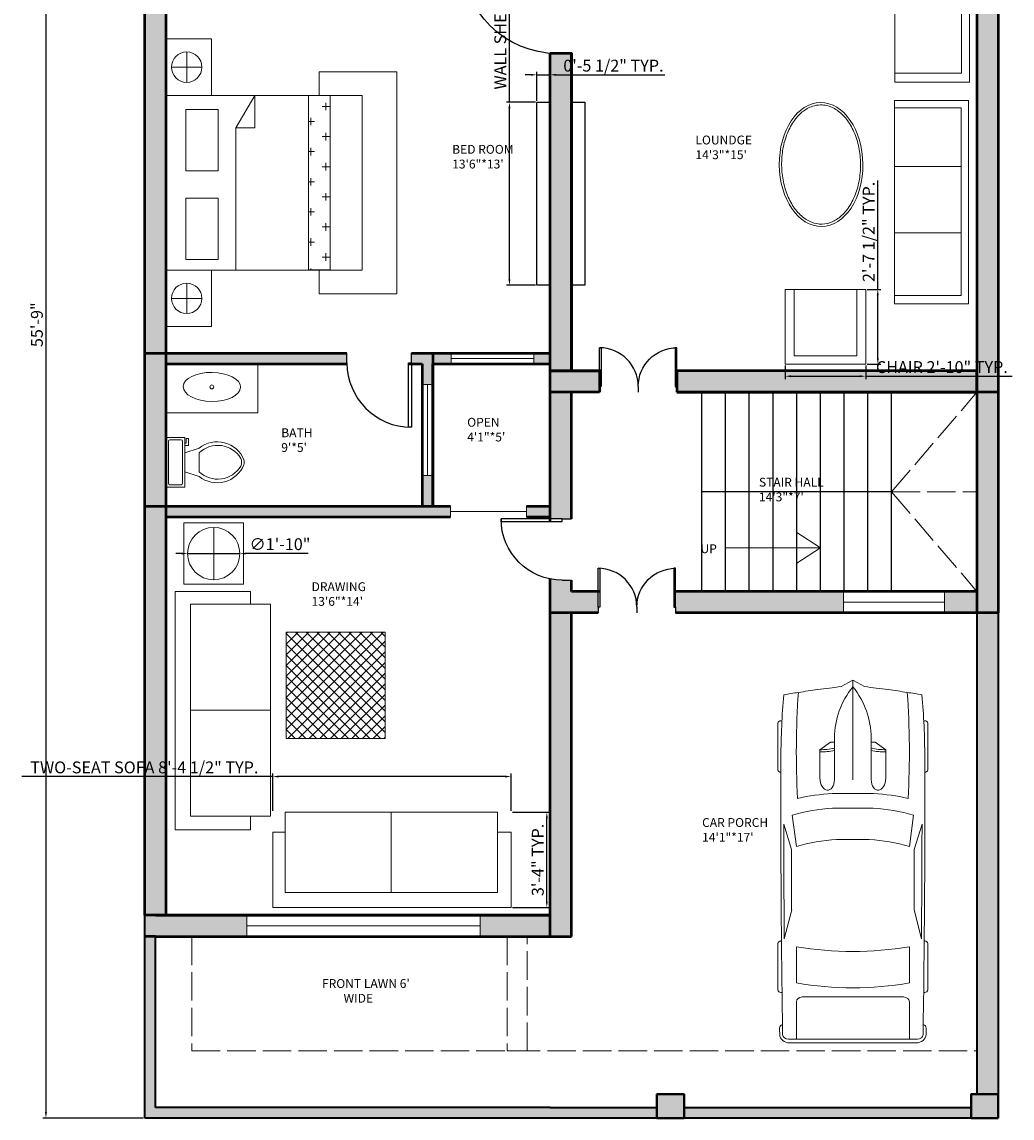
# Model space of a CAD drawing. Units: inches. Extents: x 1864 to 2313, y 963 to 1675.
# Tile 1 of 2: x 1864 to 2282, y 963 to 1425. Entities that reach past the tile are written whole.
import ezdxf

# ---------------------------------------------------------------- set-up
doc = ezdxf.new("R2010")
doc.units = ezdxf.units.IN
doc.linetypes.add('ACAD_ISO02W100', pattern=[15, 12, -3])
for name, color, linetype, lineweight in [('A-ANNO-DIMS', 210, 'Continuous', 18), ('A-ANNO-SYMB', 90, 'Continuous', 18), ('A-AREA-IDEN', 210, 'Continuous', 18), ('A-COLS', 7, 'Continuous', 40), ('A-FLOR-CASE', 230, 'Continuous', 25), ('A-FLOR-FIXT', 40, 'Continuous', 18), ('A-FLOR-OVHD', 142, 'ACAD_ISO02W100', 18), ('A-FLOR-STRS', 90, 'Continuous', 25), ('A-FLOR-STRS-HIDN', 90, 'ACAD_ISO02W100', 18), ('A-FURN-PATT', 40, 'Continuous', 13), ('A-SITE-VEHC', 230, 'Continuous', 13), ('A-SITE-WALL', 7, 'Continuous', 35), ('A-WALL-PATT', 142, 'Continuous', 13), ('door', 50, 'Continuous', 25), ('fur', 40, 'Continuous', 18), ('text', 210, 'Continuous', 18), ('wall', 7, 'Continuous', 50), ('wind', 201, 'Continuous', 20)]:
    doc.layers.add(name, color=color, linetype=linetype, lineweight=lineweight)
doc.styles.get("Standard").update_dxf_attribs({"font": 'arial.ttf'})
doc.dimstyles.new('ISO-25', dxfattribs={"dimtxt": 5, "dimasz": 2.5, "dimexe": 1.25, "dimexo": 0.625, "dimtad": 1, "dimdec": 0, "dimlunit": 4, "dimtxsty": 'Standard', "dimcen": 2.5, "dimadec": 0, "dimazin": 0, "dimtfac": 1, "dimtdec": 0, "dimtmove": 0, "dimatfit": 3, "dimfxl": 1, "dimarcsym": 0})

# ---------------------------------------------------------------- blocks, each defined once
blk = doc.blocks.new('*U6')
for p, q in [((21.1, 37.41), (21.1, 36.83)), ((46.55, 38.89), (22.35, 38.89)), ((47.8, 37.39), (47.8, 37.41)), ((87.99, 31.87), (74.76, 35.92)), ((134.31, 35.6), (119.29, 31.78)), ((135.45, 37.07), (135.45, 37.41)), ((136.7, 38.89), (160.9, 38.89)), ((162.15, 37.41), (162.15, 36.77)), ((70.03, 31.54), (86.41, 29.35)), ((138.42, 29.35), (157.25, 29.35)), ((186.47, 29.35), (167.01, 29.35)), ((186.47, -33.5), (186.47, 33.5)), ((188.4, -32.76), (188.4, 32.76)), ((164.52, 26.39), (164.52, -26.39)), ((32.27, 11.63), (36.13, 17.17)), ((36.13, 17.17), (50.94, 17.17)), ((3.27, 6.13), (0.1, 0.41)), ((29.77, 9.51), (51.68, 9.51)), ((32.12, 9.51), (32.12, 11.15)), ((58.92, -10.77), (58.92, 10.77)), ((66.55, -10.53), (66.55, 10.53)), ((82.74, 8.5), (82.74, -8.5)), ((186.47, -10.53), (186.47, 10.53)), ((0, 0), (51.68, 0)), ((0.1, -0.41), (3.27, -6.13)), ((29.77, -9.51), (51.68, -9.51)), ((32.12, -9.51), (32.12, -11.15)), ((32.27, -11.63), (36.13, -17.17)), ((36.13, -17.17), (50.94, -17.17)), ((86.41, -29.35), (70.03, -31.54)), ((87.99, -31.87), (74.76, -35.92)), ((134.31, -35.6), (119.29, -31.78)), ((157.25, -29.35), (138.42, -29.35)), ((167.01, -29.35), (186.47, -29.35)), ((21.1, -37.41), (21.1, -36.83)), ((46.55, -38.89), (22.35, -38.89)), ((47.8, -37.39), (47.8, -37.41)), ((135.45, -37.07), (135.45, -37.41)), ((136.7, -38.89), (160.9, -38.89)), ((162.15, -37.41), (162.15, -36.77))]:
    blk.add_line(p, q)
for centre, major_axis, ratio, start_param, end_param in [((266.03, -27.52), (0, 313.31), 0.842304, 1.367076, 1.39176), ((41.19, -490.86), (0, 528.23), 0.842304, 0.00281, 0.075598), ((22.35, 37.41), (0, -1.48), 0.842304, 3.141593, 4.712389), ((64.48, -10555.62), (0, 10593.03), 0.842304, -0.013397, 0.002797), ((46.55, 37.41), (0, 1.48), 0.842304, -1.570796, 0), ((64.48, -10555.62), (0, -10591.55), 0.842304, 3.133765, 3.140441), ((136.7, 37.41), (0, -1.48), 0.842304, 3.141593, 4.712389), ((160.9, 37.41), (0, 1.48), 0.842304, -1.570796, 0), ((180.63, 35.84), (0, 2.22), 0.842304, -0.013017, 1.249894), ((64.48, -10556.36), (0, 10595.31), 0.842304, -0.013397, -0.013017), ((183.98, 33.5), (0, -2.96), 0.842304, 1.570796, 3.128196), ((183.98, 32.76), (0, -5.25), 0.842304, 1.570796, 3.128196), ((37.47, -593.96), (0, -623.33), 0.842304, 3.096046, 3.200911), ((134.4, 5.39), (0, -89.78), 0.842304, 4.449482, 4.652344), ((135.29, 5.39), (0, 81.77), 0.842304, 1.245306, 1.50788), ((149.6, 2.8), (0, -79.58), 0.842304, 4.372215, 4.640744), ((95.79, -3666.35), (0, -3698.24), 0.842304, 3.134049, 3.144098), ((17.08, 0), (0, 147.02), 0.842304, 4.511394, 4.913384), ((35.91, 0), (0, 147.02), 0.842304, 4.511394, 4.913384), ((167.01, 26.39), (0, 2.96), 0.842304, 0, 1.570796), ((259.18, -27.52), (0, -305.3), 0.842304, 4.528606, 4.561838), ((-204.49, 52.4), (0, -250.96), 0.842304, 1.385369, 1.434372), ((13.04, 17.01), (0, 27.42), 0.842304, 4.435146, 4.718221), ((14.2, 17.01), (0, 27.42), 0.842304, 4.435146, 4.718221), ((50.79, 13.34), (6.34, -0.36), 0.603834, -1.395552, 1.581315), ((32.75, 11.15), (0, 0.74), 0.842304, 0.879714, 1.570796), ((29.77, -46.66), (0, 56.17), 0.842304, 0, 0.590319), ((0.62, 0), (0, -0.74), 0.842304, 4.131459, 5.293319), ((29.77, 46.66), (0, 56.17), 0.842304, 2.551274, 3.141593), ((-204.49, -52.4), (0, 250.96), 0.842304, -1.434372, -1.385369), ((32.75, -11.15), (0, -0.74), 0.842304, 4.712389, 5.403472), ((13.04, -17.01), (0, -27.42), 0.842304, 1.564964, 1.848039), ((14.2, -17.01), (0, -27.42), 0.842304, 1.564964, 1.848039), ((134.4, -5.39), (0, -89.78), 0.842304, -1.510751, -1.307889), ((135.29, -5.39), (0, -81.77), 0.842304, -1.50788, -1.245306), ((149.6, -2.8), (0, -79.58), 0.842304, -1.499151, -1.230623), ((259.18, 27.52), (0, 305.3), 0.842304, 1.721348, 1.754579), ((266.03, 27.52), (0, 313.31), 0.842304, 1.749832, 1.774517), ((37.47, 593.96), (0, -623.33), 0.842304, -0.059319, 0.045547), ((167.01, -26.39), (0, -2.96), 0.842304, 4.712389, 6.283185), ((95.79, 3666.35), (0, -3698.24), 0.842304, -0.002505, 0.007544), ((183.98, -33.5), (0, 2.96), 0.842304, 3.15499, 4.712389), ((183.98, -32.76), (0, -5.25), 0.842304, 0.013397, 1.570796), ((41.19, 490.86), (0, -528.23), 0.842304, -0.075598, -0.00281), ((22.35, -37.41), (0, 1.48), 0.842304, 1.570796, 3.141593), ((64.48, 10555.62), (0, 10593.03), 0.842304, 3.138796, 3.15499), ((46.55, -37.41), (0, -1.48), 0.842304, 0, 1.570796), ((64.48, 10555.62), (0, -10591.55), 0.842304, 0.001152, 0.007828), ((136.7, -37.41), (0, -1.48), 0.842304, -1.570796, 0), ((160.9, -37.41), (0, 1.48), 0.842304, 3.141593, 4.712389), ((180.63, -35.84), (0, -2.22), 0.842304, -1.249894, 0.013017), ((64.48, 10556.36), (0, 10595.31), 0.842304, 3.15461, 3.15499)]:
    blk.add_ellipse(centre, major_axis=major_axis, ratio=ratio, start_param=start_param, end_param=end_param)
at = {"extrusion": (0, 0, -1)}
blk.add_ellipse((50.79, -13.34), major_axis=(6.34, 0.36), ratio=0.603834, start_param=-1.395552, end_param=1.581315, dxfattribs=at)
blk = doc.blocks.new('*U2')
for p, q in [((0, 0), (0, -6)), ((40, 0), (40, -6))]:
    blk.add_line(p, q)
blk.add_lwpolyline([(0, 0), (0, 40), (1.75, 40), (1.75, 0)], close=True)
blk.add_arc((0, 0), 40, 0, 90)
blk = doc.blocks.new('*U4')
for p, q in [((9.5, -6), (9.5, -2)), ((-10, -8.5), (-8, -8.5)), ((-10, -9.5), (-10, -8.5)), ((-8, -8.5), (-8, -8)), ((-7, -8), (-7, -9.5)), ((-4, -8), (-6, -14)), ((4, -8), (6, -14)), ((-7, -9.5), (-10, -9.5)), ((4, -14), (-4, -14))]:
    blk.add_line(p, q)
blk.add_lwpolyline([(10.5, -8), (10.5, 0), (-10.5, 0), (-10.5, -8)], close=True)
for points in [[(-9.5, -2), (-9.5, -6)], [(8.5, -1), (-8.5, -1)], [(-8.5, -7), (8.5, -7)]]:
    blk.add_lwpolyline(points)
for centre, radius, start, end in [((-8.62, -1.88), 0.884, 81.8699, 188.1301), ((8.62, -1.88), 0.884, 351.8699, 98.1301), ((-8.62, -6.12), 0.884, 171.8699, 278.1301), ((8.62, -6.12), 0.884, 261.8699, 8.1301), ((3.52, -21.58), 12.17, 141.4691, 247.9714), ((4.2, -21.82), 11.33, 136.3677, 238.9468), ((-3.52, -21.58), 12.17, 292.0284, 38.5307), ((-4.2, -21.82), 11.33, 301.053, 43.6321), ((0, -27.88), 4, 245.7318, 294.2682), ((0, -29), 4, 254.8605, 285.1395)]:
    blk.add_arc(centre, radius, start, end)
blk = doc.blocks.new('*D10')
at = {"layer": 'A-ANNO-DIMS', "color": 0, "lineweight": -2, "transparency": 16777216}
for p, q in [((1915.33, 1632.16), (1873.06, 1632.16)), ((1874.31, 1629.66), (1874.31, 965.66)), ((1915.33, 963.16), (1873.06, 963.16))]:
    blk.add_line(p, q, dxfattribs=at)
at = {"layer": 'A-ANNO-DIMS', "color": 0, "lineweight": 100, "transparency": 16777216}
for points in [[(1873.89, 1629.66), (1874.73, 1629.66), (1874.31, 1632.16)], [(1873.89, 965.66), (1874.73, 965.66), (1874.31, 963.16)]]:
    blk.add_solid(points, dxfattribs=at)
at = {"layer": 'Defpoints', "color": 0, "lineweight": 100, "transparency": 16777216}
for p in [(1915.95, 1632.16), (1874.31, 963.16), (1915.95, 963.16)]:
    blk.add_point(p, dxfattribs=at)
at = {"layer": 'A-ANNO-DIMS', "color": 0, "transparency": 16777216, "insert": (1871.13, 1297.66), "char_height": 5, "attachment_point": 5, "rotation": 90}
blk.add_mtext('55\'-9"', dxfattribs=at)
blk = doc.blocks.new('BED-DOUBLE')
for p, q in [((10, 67.81), (70, 67.81)), ((70, 67.81), (70, 59.9)), ((83.6, 59.9), (70, 67.81)), ((70, 59.9), (83.6, 59.9)), ((5, 32.66), (0, 32.66)), ((0, 32.66), (0, 0)), ((10, 32.66), (5, 32.66)), ((83.6, 32.66), (93.6, 32.66)), ((93.6, 32.66), (93.6, 0)), ((0, 0), (93.6, 0))]:
    blk.add_line(p, q)
for points in [[(10, 97.3), (83.6, 97.3), (83.6, 14.55), (10, 14.55)], [(14.44, 88.9), (40.24, 88.9), (40.24, 75.28), (14.44, 75.28)], [(51.82, 88.9), (77.62, 88.9), (77.62, 75.28), (51.82, 75.28)]]:
    blk.add_lwpolyline(points, close=True)
blk = doc.blocks.new('TABLE-BEDSIDE')
for p, q in [((11.93, 4.03), (11.93, 16.85)), ((5.53, 10.44), (18.34, 10.44))]:
    blk.add_line(p, q)
blk.add_lwpolyline([(0, 19.17), (23.88, 19.17), (23.88, 0), (0, 0)], close=True)
blk.add_circle((11.93, 10.44), 6.41)
blk = doc.blocks.new('SOFA-TWO-SEAT')
for p, q in [((0, 0), (0, 100.52)), ((31.78, 100.52), (0, 100.52)), ((31.78, 95.26), (31.78, 100.52)), ((40.15, 50.52), (6.4, 50.52)), ((31.78, 5.79), (31.78, 0)), ((31.78, 0), (0, 0))]:
    blk.add_line(p, q)
blk.add_lwpolyline([(6.4, 95.26), (40.15, 95.26), (40.15, 5.79), (6.4, 5.79)], close=True)
blk = doc.blocks.new('LOUNGE-CHAIR')
for p, q in [((3.79, 31.54), (0, 31.54)), ((0, 31.54), (0, 0)), ((3.79, 3.47), (3.79, 31.54)), ((30.24, 31.54), (33.95, 31.54)), ((33.95, 31.54), (33.95, 0)), ((0, 0), (33.95, 0))]:
    blk.add_line(p, q)
blk.add_lwpolyline([(3.79, 31.54), (30.24, 31.54), (30.24, 3.47), (3.79, 3.47)])
blk = doc.blocks.new('BASIN-OVAL')
blk.add_circle((12.11, 6.1), 0.811)
blk.add_ellipse((12.11, 6.1), major_axis=(12.1, -0.16), ratio=0.504372)
blk = doc.blocks.new('WALL-SHELF')
blk.add_lwpolyline([(0, 77.17), (5.6, 77.17), (5.6, 0), (0, 0)], close=True)
blk = doc.blocks.new('*D24')
at = {"layer": 'A-ANNO-DIMS', "color": 0, "lineweight": -2, "transparency": 16777216}
for p, q in [((1969.95, 1107.15), (1864.18, 1107.15)), ((1969.95, 1092.7), (1969.95, 1108.4)), ((2067.97, 1107.15), (1972.45, 1107.15)), ((2070.47, 1092.7), (2070.47, 1108.4))]:
    blk.add_line(p, q, dxfattribs=at)
at = {"layer": 'A-ANNO-DIMS', "color": 0, "lineweight": 100, "transparency": 16777216}
for points in [[(1972.45, 1107.57), (1972.45, 1106.74), (1969.95, 1107.15)], [(2067.97, 1107.57), (2067.97, 1106.74), (2070.47, 1107.15)]]:
    blk.add_solid(points, dxfattribs=at)
at = {"layer": 'Defpoints', "color": 0, "lineweight": 100, "transparency": 16777216}
for p in [(1969.95, 1107.15), (1969.95, 1092.07), (2070.47, 1092.07)]:
    blk.add_point(p, dxfattribs=at)
at = {"layer": 'A-ANNO-DIMS', "color": 0, "transparency": 16777216, "insert": (1915.81, 1110.36), "char_height": 5, "attachment_point": 5}
blk.add_mtext('TWO-SEAT SOFA 8\'-4 1/2" TYP.', dxfattribs=at)
blk = doc.blocks.new('*D25')
at = {"layer": 'A-ANNO-DIMS', "color": 0, "lineweight": -2, "transparency": 16777216}
for p, q in [((2071.09, 1092.07), (2086.8, 1092.07)), ((2085.55, 1054.43), (2085.55, 1089.57)), ((2071.09, 1051.93), (2086.8, 1051.93))]:
    blk.add_line(p, q, dxfattribs=at)
at = {"layer": 'A-ANNO-DIMS', "color": 0, "lineweight": 100, "transparency": 16777216}
for points in [[(2085.13, 1089.57), (2085.96, 1089.57), (2085.55, 1092.07)], [(2085.13, 1054.43), (2085.96, 1054.43), (2085.55, 1051.93)]]:
    blk.add_solid(points, dxfattribs=at)
at = {"layer": 'Defpoints', "color": 0, "lineweight": 100, "transparency": 16777216}
for p in [(2070.47, 1092.07), (2085.55, 1092.07), (2070.47, 1051.93)]:
    blk.add_point(p, dxfattribs=at)
at = {"layer": 'A-ANNO-DIMS', "color": 0, "transparency": 16777216, "insert": (2082.37, 1072), "char_height": 5, "attachment_point": 5, "rotation": 90}
blk.add_mtext('3\'-4" TYP.', dxfattribs=at)
blk = doc.blocks.new('*D26')
at = {"layer": 'A-ANNO-DIMS', "color": 0, "lineweight": -2, "transparency": 16777216}
for p, q in [((2186.08, 1280.4), (2186.08, 1274.68)), ((2220.03, 1280.4), (2220.03, 1274.68)), ((2188.58, 1275.93), (2217.53, 1275.93)), ((2220.03, 1275.93), (2281.76, 1275.93))]:
    blk.add_line(p, q, dxfattribs=at)
at = {"layer": 'A-ANNO-DIMS', "color": 0, "lineweight": 100, "transparency": 16777216}
for points in [[(2188.58, 1276.35), (2188.58, 1275.52), (2186.08, 1275.93)], [(2217.53, 1276.35), (2217.53, 1275.52), (2220.03, 1275.93)]]:
    blk.add_solid(points, dxfattribs=at)
at = {"layer": 'Defpoints', "color": 0, "lineweight": 100, "transparency": 16777216}
for p in [(2186.08, 1281.02), (2220.03, 1281.02), (2220.03, 1275.93)]:
    blk.add_point(p, dxfattribs=at)
at = {"layer": 'A-ANNO-DIMS', "color": 0, "transparency": 16777216, "insert": (2252.15, 1279.14), "char_height": 5, "attachment_point": 5}
blk.add_mtext('CHAIR 2\'-10" TYP.', dxfattribs=at)
blk = doc.blocks.new('*D27')
at = {"layer": 'A-ANNO-DIMS', "color": 0, "lineweight": -2, "transparency": 16777216}
for p, q in [((2225.13, 1312.56), (2225.13, 1358.53)), ((2220.66, 1312.56), (2226.38, 1312.56)), ((2225.13, 1283.52), (2225.13, 1310.06)), ((2220.66, 1281.02), (2226.38, 1281.02))]:
    blk.add_line(p, q, dxfattribs=at)
at = {"layer": 'A-ANNO-DIMS', "color": 0, "lineweight": 100, "transparency": 16777216}
for points in [[(2224.71, 1310.06), (2225.54, 1310.06), (2225.13, 1312.56)], [(2224.71, 1283.52), (2225.54, 1283.52), (2225.13, 1281.02)]]:
    blk.add_solid(points, dxfattribs=at)
at = {"layer": 'Defpoints', "color": 0, "lineweight": 100, "transparency": 16777216}
for p in [(2220.03, 1312.56), (2225.13, 1312.56), (2220.03, 1281.02)]:
    blk.add_point(p, dxfattribs=at)
at = {"layer": 'A-ANNO-DIMS', "color": 0, "transparency": 16777216, "insert": (2221.92, 1336.8), "char_height": 5, "attachment_point": 5, "rotation": 90}
blk.add_mtext('2\'-7 1/2" TYP.', dxfattribs=at)
blk = doc.blocks.new('*D30')
at = {"layer": 'A-ANNO-DIMS', "color": 0, "lineweight": -2, "transparency": 16777216}
for p, q in [((2069.78, 1391.45), (2069.78, 1471.3)), ((2080.73, 1391.45), (2068.53, 1391.45)), ((2069.78, 1316.78), (2069.78, 1388.95)), ((2080.73, 1314.28), (2068.53, 1314.28))]:
    blk.add_line(p, q, dxfattribs=at)
at = {"layer": 'A-ANNO-DIMS', "color": 0, "lineweight": 100, "transparency": 16777216}
for points in [[(2069.36, 1388.95), (2070.19, 1388.95), (2069.78, 1391.45)], [(2069.36, 1316.78), (2070.19, 1316.78), (2069.78, 1314.28)]]:
    blk.add_solid(points, dxfattribs=at)
at = {"layer": 'Defpoints', "color": 0, "lineweight": 100, "transparency": 16777216}
for p in [(2069.78, 1391.45), (2081.35, 1391.45), (2081.35, 1314.28)]:
    blk.add_point(p, dxfattribs=at)
at = {"layer": 'A-ANNO-DIMS', "color": 0, "transparency": 16777216, "insert": (2066.57, 1432.63), "char_height": 5, "attachment_point": 5, "rotation": 90}
blk.add_mtext('WALL SHELF 6\'-5" TYP.', dxfattribs=at)
blk = doc.blocks.new('*D31')
at = {"layer": 'A-ANNO-DIMS', "color": 0, "lineweight": -2, "transparency": 16777216}
for p, q in [((2078.85, 1403.03), (2076.35, 1403.03)), ((2081.35, 1392.08), (2081.35, 1404.28)), ((2081.35, 1403.03), (2086.95, 1403.03)), ((2086.95, 1392.08), (2086.95, 1404.28)), ((2089.45, 1403.03), (2135.33, 1403.03))]:
    blk.add_line(p, q, dxfattribs=at)
at = {"layer": 'A-ANNO-DIMS', "color": 0, "lineweight": 100, "transparency": 16777216}
for points in [[(2078.85, 1403.44), (2078.85, 1402.61), (2081.35, 1403.03)], [(2089.45, 1403.44), (2089.45, 1402.61), (2086.95, 1403.03)]]:
    blk.add_solid(points, dxfattribs=at)
at = {"layer": 'Defpoints', "color": 0, "lineweight": 100, "transparency": 16777216}
for p in [(2086.95, 1403.03), (2081.35, 1391.45), (2086.95, 1391.45)]:
    blk.add_point(p, dxfattribs=at)
at = {"layer": 'A-ANNO-DIMS', "color": 0, "transparency": 16777216, "insert": (2113.64, 1406.24), "char_height": 5, "attachment_point": 5}
blk.add_mtext('0\'-5 1/2" TYP.', dxfattribs=at)
blk = doc.blocks.new('*D34')
at = {"layer": 'A-ANNO-DIMS', "color": 0, "lineweight": -2, "transparency": 16777216}
for p, q in [((1931.54, 1201.15), (1929.04, 1201.15)), ((1934.04, 1201.15), (1956.09, 1201.15)), ((1984.95, 1201.15), (1958.59, 1201.15))]:
    blk.add_line(p, q, dxfattribs=at)
at = {"layer": 'A-ANNO-DIMS', "color": 0, "lineweight": 100, "transparency": 16777216}
for points in [[(1931.54, 1201.56), (1931.54, 1200.73), (1934.04, 1201.15)], [(1958.59, 1201.56), (1958.59, 1200.73), (1956.09, 1201.15)]]:
    blk.add_solid(points, dxfattribs=at)
at = {"layer": 'Defpoints', "color": 0, "lineweight": 100, "transparency": 16777216}
for p in [(1934.04, 1201.15), (1956.09, 1201.15)]:
    blk.add_point(p, dxfattribs=at)
at = {"layer": 'A-ANNO-DIMS', "color": 0, "transparency": 16777216, "insert": (1973.02, 1204.47), "char_height": 5, "attachment_point": 5, "rotation": 359.9997}
blk.add_mtext('∅1\'-10"', dxfattribs=at)

msp = doc.modelspace()

# ---------------------------------------------------------------- hatches: boundary and pattern name
at = {"layer": 'A-FURN-PATT'}
h = msp.add_hatch(dxfattribs=at)
h.set_pattern_fill('CROSS', color=256, angle=90)
h.set_pattern_definition([(90, (3548.109, -701.066), (-6.35, 6.35), [3.175, -9.525]), (180, (3549.697, -699.4784), (-6.35, -6.35), [3.175, -9.525])])
h.paths.add_polyline_path([(1994.15, 1394.32), (1985.02, 1394.32), (1985.02, 1320.73), (1994.15, 1320.73)])
h = msp.add_hatch(dxfattribs=at)
h.set_pattern_fill('ANSI37', color=256)
h.paths.add_polyline_path([(2017.33, 1167.99), (1975.66, 1167.99), (1975.66, 1123.22), (2017.33, 1123.22)])
at = {"layer": 'A-WALL-PATT'}
h = msp.add_hatch(color=256, dxfattribs=at)
h.dxf.hatch_style = 1
h.paths.add_polyline_path([(1975.95, 1632.16), (1961.64, 1632.16), (1961.64, 1623.16), (1971.45, 1623.16), (1975.95, 1623.16)])
h.paths.add_polyline_path([(2021.79, 1632.16), (1989.45, 1632.16), (1975.95, 1632.16), (1975.95, 1623.16), (1984.95, 1623.16), (1989.45, 1623.16), (2021.79, 1623.16)])
h.paths.add_polyline_path([(2161.95, 1632.16), (2126.93, 1632.16), (2126.93, 1623.16), (2157.45, 1623.16), (2161.95, 1623.16)])
h.paths.add_polyline_path([(2275.95, 1632.16), (2258.45, 1632.16), (2258.45, 1623.16), (2266.95, 1623.16), (2266.95, 1475.18, -0.040334), (2266.95, 1472.91), (2266.95, 1467.16), (2266.95, 1458.16), (2266.95, 1278.16), (2266.95, 1269.16), (2275.95, 1269.16), (2275.95, 1458.16)])
h.paths.add_polyline_path([(2161.95, 1623.16), (2157.45, 1623.16), (2157.45, 1467.16), (2154.26, 1467.16), (2154.26, 1464.16), (2154.26, 1458.16), (2161.95, 1458.16)])
h.paths.add_polyline_path([(2202.62, 1632.16), (2198.67, 1632.16), (2198.67, 1627.01, -0.028105), (2198.46, 1623.16), (2202.62, 1623.16)])
h.paths.add_polyline_path([(2164.34, 1627.01), (2164.34, 1632.16), (2161.95, 1632.16), (2161.95, 1623.16), (2164.34, 1623.16)])
h.paths.add_polyline_path([(1930.16, 1632.16), (1929.45, 1632.16), (1915.95, 1632.16), (1915.95, 1458.16), (1924.95, 1458.16), (1924.95, 1623.16), (1930.16, 1623.16)])
h.paths.add_polyline_path([(1924.95, 1441.66), (1924.95, 1458.16), (1915.95, 1458.16), (1915.95, 1285.66), (1924.95, 1285.66)])
h.paths.add_polyline_path([(2044.94, 1221.16), (2037.45, 1221.16), (1924.95, 1221.16), (1924.95, 1216.66), (2044.94, 1216.66)])
h.paths.add_polyline_path([(2037.45, 1234.15), (2032.95, 1234.15), (2032.95, 1221.16), (2037.45, 1221.16)])
h.paths.add_polyline_path([(2086.95, 1221.16), (2076.95, 1221.16), (2076.95, 1216.66), (2086.95, 1216.66)])
h.paths.add_polyline_path([(2107.14, 1185.16), (2095.95, 1185.16), (2095.95, 1189.94), (2092.08, 1189.94, -0.049915), (2086.95, 1190.46), (2086.95, 1176.16), (2107.14, 1176.16), (2107.14, 1178.61)])
h.paths.add_polyline_path([(2095.95, 1176.16), (2086.95, 1176.16), (2086.95, 1056.16), (2086.95, 1039.66), (2095.95, 1039.66), (2095.95, 1056.16)])
h.paths.add_polyline_path([(2086.95, 1048.66), (2057.44, 1048.66), (2057.44, 1039.66), (2086.95, 1039.66)])
h.paths.add_polyline_path([(1959.08, 1048.66), (1915.95, 1048.66), (1915.95, 1039.66), (1920.45, 1039.66), (1959.08, 1039.66)])
h.paths.add_polyline_path([(1924.95, 1216.66), (1924.95, 1221.16), (1915.95, 1221.16), (1915.95, 1048.66), (1924.95, 1048.66)])
h.paths.add_polyline_path([(1924.95, 1281.16), (1924.95, 1285.66), (1915.95, 1285.66), (1915.95, 1221.16), (1924.95, 1221.16)])
h.paths.add_polyline_path([(2037.45, 1285.66), (2028.44, 1285.66), (2028.44, 1281.58), (2028.44, 1281.16), (2032.95, 1281.16), (2032.95, 1272.41), (2037.45, 1272.41)])
h.paths.add_polyline_path([(2045.26, 1285.66), (2037.45, 1285.66), (2037.45, 1281.16), (2045.26, 1281.16)])
h.paths.add_polyline_path([(2086.95, 1285.66), (2080.03, 1285.66), (2080.03, 1281.16), (2086.95, 1281.16)])
h.paths.add_polyline_path([(2095.95, 1269.16), (2086.95, 1269.16), (2086.95, 1215.79), (2092.08, 1215.79), (2095.95, 1215.79)])
h = msp.add_hatch(color=256, dxfattribs=at)
h.dxf.hatch_style = 1
h.paths.add_polyline_path([(2266.95, 1278.16), (2140.44, 1278.16), (2140.44, 1271.61), (2140.44, 1269.16), (2266.95, 1269.16)])
h.paths.add_polyline_path([(2107.74, 1278.16), (2086.95, 1278.16), (2086.95, 1269.16), (2107.74, 1269.16), (2107.74, 1271.61)])
h.paths.add_polyline_path([(2095.95, 1412.1), (2086.95, 1412.1), (2086.95, 1278.16), (2095.95, 1278.16)])
h = msp.add_hatch(color=256, dxfattribs=at)
h.dxf.hatch_style = 1
h.paths.add_polyline_path([(2131.95, 967.66), (2086.95, 967.66), (1920.45, 967.66), (1920.45, 1039.66), (1915.95, 1039.66), (1915.95, 963.16), (2086.95, 963.16), (2131.95, 963.16)])
h.paths.add_polyline_path([(2143.4, 973.21), (2131.95, 973.21), (2131.95, 963.16), (2143.4, 963.16)])
h.paths.add_polyline_path([(2264.5, 967.66), (2143.4, 967.66), (2143.4, 963.16), (2264.5, 963.16)])
h.paths.add_polyline_path([(2275.95, 973.21), (2264.5, 973.21), (2264.5, 963.16), (2275.95, 963.16)])
h.paths.add_polyline_path([(2275.95, 1176.16), (2266.95, 1176.16), (2266.95, 973.21), (2275.95, 973.21)])
h.paths.add_polyline_path([(2210.63, 1185.16), (2139.85, 1185.16), (2139.85, 1178.61), (2139.85, 1176.16), (2210.63, 1176.16)])
h.paths.add_polyline_path([(2266.95, 1185.16), (2253.22, 1185.16), (2253.22, 1176.16), (2266.95, 1176.16)])
h.paths.add_polyline_path([(2275.95, 1269.16), (2266.95, 1269.16), (2266.95, 1185.16), (2266.95, 1176.16), (2275.95, 1176.16)])
h.paths.add_polyline_path([(2001.26, 1285.66), (1924.95, 1285.66), (1924.95, 1281.16), (1963.64, 1281.16), (2001.27, 1281.16, -0.003893), (2001.26, 1281.58)])

# ---------------------------------------------------------------- linework, layer by layer
at = {"layer": 'A-ANNO-SYMB'}
for p, q in [((2200.95, 1203.59), (2190.95, 1210.06)), ((2160.95, 1203.59), (2200.95, 1203.59)), ((2200.95, 1203.59), (2190.95, 1197.13))]:
    msp.add_line(p, q, dxfattribs=at)
at = {"layer": 'A-COLS'}
for points in [[(2143.4, 963.16), (2131.95, 963.16), (2131.95, 973.21), (2143.4, 973.21)], [(2275.95, 963.16), (2264.5, 963.16), (2264.5, 973.21), (2275.95, 973.21)]]:
    msp.add_lwpolyline(points, close=True, dxfattribs=at)
at = {"layer": 'A-FLOR-FIXT'}
msp.add_lwpolyline([(1924.95, 1281.16), (1963.64, 1281.16), (1963.64, 1260.54), (1924.95, 1260.54)], close=True, dxfattribs=at)
at = {"layer": 'A-FLOR-OVHD'}
for p, q in [((1935.8, 1039.66), (1935.8, 991.47)), ((1935.8, 991.47), (2266.95, 991.47))]:
    msp.add_line(p, q, dxfattribs=at)
msp.add_lwpolyline([(2077.24, 1039.66), (2068.83, 1039.66), (2068.83, 991.47), (2077.24, 991.47)], close=True, dxfattribs=at)
at = {"layer": 'A-FLOR-STRS'}
for p, q in [((2150.95, 1185.16), (2150.95, 1269.16)), ((2160.95, 1185.16), (2160.95, 1269.16)), ((2170.95, 1185.16), (2170.95, 1269.16)), ((2180.95, 1185.16), (2180.95, 1269.16)), ((2190.95, 1185.16), (2190.95, 1269.16)), ((2200.95, 1185.16), (2200.95, 1269.16)), ((2210.95, 1185.16), (2210.95, 1269.16)), ((2220.95, 1185.16), (2220.95, 1269.16)), ((2230.95, 1185.16), (2230.95, 1269.16)), ((2173.41, 1227.16), (2150.95, 1227.16)), ((2230.95, 1227.16), (2173.41, 1227.16))]:
    msp.add_line(p, q, dxfattribs=at)
at = {"layer": 'A-FLOR-STRS-HIDN'}
for q in [(2266.95, 1269.16), (2266.95, 1227.16), (2266.95, 1185.16)]:
    msp.add_line((2230.95, 1227.16), q, dxfattribs=at)
at = {"layer": 'A-SITE-WALL'}
for p, q in [((2266.95, 1176.16), (2266.95, 973.21)), ((2275.95, 1176.16), (2275.95, 963.16)), ((1915.95, 963.16), (1915.95, 1048.66)), ((1920.45, 967.66), (1920.45, 1039.66)), ((2086.95, 967.66), (1920.45, 967.66)), ((2086.95, 967.66), (2131.95, 967.66)), ((2143.4, 967.66), (2264.5, 967.66)), ((2086.95, 963.16), (1915.95, 963.16)), ((2275.95, 963.16), (2086.95, 963.16))]:
    msp.add_line(p, q, dxfattribs=at)
at = {"layer": 'fur'}
for p, q in [((2232.19, 1389.06), (2232.19, 1392.26)), ((2232.19, 1392.26), (2263.36, 1392.26)), ((2263.36, 1306.47), (2263.36, 1392.26)), ((2232.19, 1364.33), (2260.26, 1364.33)), ((2232.19, 1336.38), (2260.26, 1336.38)), ((2232.19, 1309.93), (2232.19, 1306.47)), ((2232.19, 1306.47), (2263.36, 1306.47)), ((1945.06, 1190.12), (1945.06, 1212.17)), ((1934.04, 1201.15), (1956.09, 1201.15))]:
    msp.add_line(p, q, dxfattribs=at)
for points in [[(1994.15, 1320.73), (1994.15, 1394.32), (1985.02, 1394.32), (1985.02, 1320.73)], [(2260.26, 1309.93), (2232.19, 1309.93), (2232.19, 1389.06), (2260.26, 1389.06)], [(1932.45, 1188.21), (1957.68, 1188.21), (1957.68, 1214.08), (1932.45, 1214.08)], [(1975.66, 1123.22), (2017.33, 1123.22), (2017.33, 1167.99), (1975.66, 1167.99)]]:
    msp.add_lwpolyline(points, close=True, dxfattribs=at)
msp.add_circle((1945.06, 1201.15), 11.03, dxfattribs=at)
msp.add_ellipse((2201.22, 1365.21), major_axis=(-0.23, 26.12), ratio=0.675316, dxfattribs=at)
msp.add_open_spline([(2201, 1390.33), (2199.84, 1390.32), (2198.68, 1390.13), (2196.06, 1389.26), (2194.62, 1388.45), (2191.91, 1386.25), (2190.65, 1384.85), (2188.42, 1381.56), (2187.46, 1379.67), (2185.93, 1375.56), (2185.35, 1373.33), (2184.64, 1368.71), (2184.51, 1366.32), (2184.69, 1361.58), (2185.01, 1359.23), (2186.06, 1354.75), (2186.8, 1352.62), (2188.64, 1348.76), (2189.73, 1347.03), (2192.19, 1344.1), (2193.54, 1342.91), (2196.38, 1341.12), (2197.87, 1340.54), (2200.87, 1339.99), (2202.39, 1340.03), (2205.39, 1340.74), (2206.88, 1341.42), (2209.69, 1343.39), (2211.02, 1344.69), (2213.39, 1347.81), (2214.43, 1349.64), (2216.13, 1353.67), (2216.79, 1355.88), (2217.66, 1360.49), (2217.88, 1362.9), (2217.84, 1367.71), (2217.59, 1370.11), (2216.65, 1374.71), (2215.96, 1376.91), (2214.2, 1380.93), (2213.13, 1382.74), (2210.72, 1385.84), (2209.37, 1387.12), (2206.52, 1389.07), (2205.03, 1389.73), (2202.68, 1390.25), (2201.84, 1390.34), (2201, 1390.33)], degree=3, knots=[0, 0, 0, 0, 0.21536, 0.21536, 0.495184, 0.495184, 0.775007, 0.775007, 1.054831, 1.054831, 1.334654, 1.334654, 1.614478, 1.614478, 1.894301, 1.894301, 2.174125, 2.174125, 2.453948, 2.453948, 2.733772, 2.733772, 3.013595, 3.013595, 3.293419, 3.293419, 3.576815, 3.576815, 3.86021, 3.86021, 4.143606, 4.143606, 4.427002, 4.427002, 4.710398, 4.710398, 4.993794, 4.993794, 5.27719, 5.27719, 5.560586, 5.560586, 5.843982, 5.843982, 6.127378, 6.127378, 6.283185, 6.283185, 6.283185, 6.283185], dxfattribs=at)
at = {"layer": 'wall'}
for p, q in [((1915.95, 1285.66), (1915.95, 1632.16)), ((1924.95, 1281.16), (1924.95, 1623.16)), ((2266.95, 1458.16), (2266.95, 1278.16)), ((2275.95, 1458.16), (2275.95, 1269.16)), ((1924.95, 1285.66), (1924.95, 1441.66)), ((2086.95, 1269.16), (2086.95, 1412.1)), ((2095.95, 1278.16), (2095.95, 1411.99)), ((1915.95, 1221.16), (1915.95, 1285.66)), ((1915.95, 1285.66), (2001.26, 1285.66)), ((2028.44, 1285.66), (2037.45, 1285.66)), ((2037.45, 1285.66), (2037.45, 1221.16)), ((2037.45, 1285.66), (2086.95, 1285.66)), ((1924.95, 1221.16), (1924.95, 1281.16)), ((1924.95, 1281.16), (2001.27, 1281.16)), ((2027.25, 1281.16), (2032.95, 1281.16)), ((2032.95, 1281.16), (2032.95, 1221.16)), ((2037.45, 1221.16), (2037.45, 1281.16)), ((2037.45, 1281.16), (2086.95, 1281.16)), ((2108.46, 1278.16), (2095.95, 1278.16)), ((2266.95, 1278.16), (2139.73, 1278.16)), ((2266.95, 1278.16), (2266.95, 1269.16)), ((2107.74, 1269.16), (2086.95, 1269.16)), ((2086.95, 1214.66), (2086.95, 1269.16)), ((2095.95, 1215.79), (2095.95, 1269.16)), ((2275.95, 1269.16), (2140.44, 1269.16)), ((2266.95, 1269.16), (2266.95, 1185.16)), ((2275.95, 1269.16), (2275.95, 1176.16)), ((1915.95, 1048.66), (1915.95, 1221.16)), ((1915.95, 1221.16), (2044.94, 1221.16)), ((1924.95, 1216.66), (1924.95, 1221.16)), ((2037.45, 1221.16), (2044.94, 1221.16)), ((2076.95, 1221.16), (2086.45, 1221.16)), ((2076.95, 1221.16), (2086.95, 1221.16)), ((1924.95, 1048.66), (1924.95, 1216.66)), ((1924.95, 1216.66), (2044.94, 1216.66)), ((2076.95, 1216.66), (2086.95, 1216.66)), ((2086.95, 1176.16), (2086.95, 1190.46)), ((2095.95, 1185.16), (2095.95, 1189.94)), ((2107.86, 1185.16), (2095.95, 1185.16)), ((2266.95, 1185.16), (2139.13, 1185.16)), ((2266.95, 1185.16), (2230.95, 1185.16)), ((2266.95, 1185.16), (2266.95, 1176.16)), ((2086.95, 1056.16), (2086.95, 1176.16)), ((2107.14, 1176.16), (2086.95, 1176.16)), ((2095.95, 1056.16), (2095.95, 1176.16)), ((2275.95, 1176.16), (2139.85, 1176.16)), ((2086.95, 1039.66), (2086.95, 1056.16)), ((2095.95, 1039.66), (2095.95, 1056.16)), ((2086.95, 1048.66), (1915.95, 1048.66)), ((1920.45, 1048.66), (2086.95, 1048.66)), ((1920.45, 1039.66), (1915.95, 1039.66)), ((1920.45, 1039.66), (2086.95, 1039.66)), ((2086.95, 1039.66), (2095.95, 1039.66))]:
    msp.add_line(p, q, dxfattribs=at)
for points in [[(2086.95, 1412.1), (2095.95, 1412.1), (2095.95, 1278.16), (2086.95, 1278.16)], [(2107.74, 1269.16), (2086.95, 1269.16), (2086.95, 1278.16), (2107.74, 1278.16)], [(2140.44, 1269.16), (2266.95, 1269.16), (2266.95, 1278.16), (2140.44, 1278.16)]]:
    msp.add_lwpolyline(points, close=True, dxfattribs=at)
at = {"layer": 'wind'}
for p, q in [((2045.26, 1283.41), (2080.03, 1283.41)), ((2035.2, 1234.15), (2035.2, 1272.41)), ((2044.94, 1221.16), (2044.94, 1216.66)), ((2076.95, 1221.16), (2076.95, 1216.66)), ((2044.94, 1218.91), (2076.95, 1218.91)), ((2210.63, 1180.66), (2253.22, 1180.66)), ((1959.08, 1044.16), (2057.44, 1044.16))]:
    msp.add_line(p, q, dxfattribs=at)
for points in [[(2045.26, 1285.66), (2080.03, 1285.66), (2080.03, 1281.16), (2045.26, 1281.16)], [(2032.95, 1234.15), (2037.45, 1234.15), (2037.45, 1272.41), (2032.95, 1272.41)], [(2253.22, 1185.16), (2210.63, 1185.16), (2210.63, 1176.16), (2253.22, 1176.16)], [(1959.08, 1048.66), (2057.44, 1048.66), (2057.44, 1039.66), (1959.08, 1039.66)]]:
    msp.add_lwpolyline(points, close=True, dxfattribs=at)

# ---------------------------------------------------------------- block references
at = {"layer": 'A-FLOR-CASE'}
for p in [(2081.35, 1314.28), (2095.95, 1314.28)]:
    msp.add_blockref('WALL-SHELF', p, dxfattribs=at)
at = {"layer": 'A-FLOR-FIXT'}
msp.add_blockref('BASIN-OVAL', (1932.18, 1265.33), dxfattribs=at)
at = {"layer": 'A-FLOR-FIXT', "xscale": -1, "rotation": 90}
msp.add_blockref('*U4', (1924.95, 1239.67), dxfattribs=at)
at = {"layer": 'A-SITE-VEHC', "xscale": 0.8119099939456049, "yscale": 0.8119099939456049, "zscale": 0.8119099939456049, "rotation": 270}
msp.add_blockref('*U6', (2214.61, 1147.79), dxfattribs=at)
at = {"layer": 'door', "xscale": -1, "rotation": 90}
msp.add_blockref('*U2', (2089.95, 1451.99), dxfattribs=at)
at = {"layer": 'door'}
for p, xscale, yscale, zscale, rotation in [((2028.44, 1281.58), 0.6794589674034023, 0.6794589674034023, 0.6794589674034023, 180), ((2092.08, 1215.79), -0.6462302409556835, 0.6462302409556835, 0.6462302409556835, 90)]:
    msp.add_blockref('*U2', p, dxfattribs=dict(at, xscale=xscale, yscale=yscale, zscale=zscale, rotation=rotation))
at = {"layer": 'door', "yscale": 0.4087596581747145, "zscale": 0.4087596581747145}
for p, xscale in [((2107.74, 1271.61), 0.4087596581747145), ((2140.44, 1271.61), -0.4087596581747145), ((2107.14, 1178.61), 0.4087596581747145), ((2139.85, 1178.61), -0.4087596581747145)]:
    msp.add_blockref('*U2', p, dxfattribs=dict(at, xscale=xscale))
at = {"layer": 'fur'}
for name, p, rotation in [('LOUNGE-CHAIR', (2263.85, 1399.95), 89.99999999999964), ('TABLE-BEDSIDE', (1944.12, 1394.32), 89.99999999999766), ('BED-DOUBLE', (2022.25, 1310.72), 90.00000000000259), ('TABLE-BEDSIDE', (1944.12, 1296.84), 89.9999999999994), ('SOFA-TWO-SEAT', (2070.47, 1051.93), 89.99999999999982)]:
    msp.add_blockref(name, p, dxfattribs=dict(at, rotation=rotation))
for name, p in [('LOUNGE-CHAIR', (2186.08, 1281.02)), ('SOFA-TWO-SEAT', (1928.87, 1084.64))]:
    msp.add_blockref(name, p, dxfattribs=at)

# ---------------------------------------------------------------- texts
at = {"layer": 'A-AREA-IDEN', "attachment_point": 1}
for s, insert, char_height in [('LOUNDGE\\P14\'3"*15\'', (2148.22, 1377.4), 3.726), ('BED ROOM\\P13\'6"*13\'', (2045.64, 1373.47), 3.726), ('OPEN\\P4\'1"*5\'', (2051.97, 1258.38), 3.726), ("BATH\\P9'*5'", (1973.55, 1253.95), 3.726), ('STAIR HALL\\P14\'3"*7\'', (2175.01, 1233.11), 3.726), ('DRAWING\\P13\'6"*14\'', (1986.33, 1189.07), 3.726), ('CAR PORCH\\P14\'1"*17\'', (2151.03, 1089.63), 3.726), ("FRONT LAWN 6'\\P        WIDE", (1990.72, 1021.75), 3.7259)]:
    msp.add_mtext_dynamic_manual_height_columns(s, width=46.4423, gutter_width=18.63, heights=[0], dxfattribs=dict(at, insert=insert, char_height=char_height))
at = {"layer": 'text', "insert": (2150.37, 1205.06), "char_height": 3.726, "attachment_point": 1}
msp.add_mtext_dynamic_manual_height_columns('UP', width=46.4423, gutter_width=18.63, heights=[0], dxfattribs=at)

# ---------------------------------------------------------------- dimensions: what is measured, and where the dimension line sits
at = {"layer": 'A-ANNO-DIMS'}
dim = msp.add_linear_dim(base=(1874.31, 963.16), p1=(1915.95, 1632.16), p2=(1915.95, 963.16), angle=90, dimstyle='ISO-25', override={"dimclrd": 0, "dimclre": 0, "dimclrt": 0}, dxfattribs=at)
dim.commit()
dim.dimension.update_dxf_attribs({"geometry": '*D10', "text_midpoint": (1871.13, 1297.66)})
for base, p1, p2, angle, text, picture, middle in [((2069.78, 1391.45), (2081.35, 1314.28), (2081.35, 1391.45), 90, 'WALL SHELF <> TYP.', '*D30', (2066.57, 1432.63)), ((2225.13, 1312.56), (2220.03, 1281.02), (2220.03, 1312.56), 90, '<> TYP.', '*D27', (2221.92, 1336.8)), ((1969.95, 1107.15), (2070.47, 1092.07), (1969.95, 1092.07), 180, 'TWO-SEAT SOFA <> TYP.', '*D24', (1915.81, 1110.36)), ((2085.55, 1092.07), (2070.47, 1051.93), (2070.47, 1092.07), 90, '<> TYP.', '*D25', (2082.37, 1072))]:
    dim = msp.add_linear_dim(base=base, p1=p1, p2=p2, angle=angle, text=text, dimstyle='ISO-25', override={"dimdec": 1, "dimlfac": 1, "dimrnd": 0, "dimzin": 1, "dimdsep": 46, "dimlunit": 4, "dimfrac": 2}, dxfattribs=at)
    dim.commit()
    dim.dimension.update_dxf_attribs({"geometry": picture, "text_midpoint": middle})
for base, p1, p2, text, picture, middle in [((2086.95, 1403.03), (2081.35, 1391.45), (2086.95, 1391.45), '<> TYP.', '*D31', (2113.64, 1406.24)), ((2220.0334, 1275.9323), (2186.0848, 1281.0246), (2220.0334, 1281.0246), 'CHAIR <> TYP.', '*D26', (2252.1472, 1279.1426))]:
    dim = msp.add_linear_dim(base=base, p1=p1, p2=p2, text=text, dimstyle='ISO-25', override={"dimdec": 1, "dimlfac": 1, "dimrnd": 0, "dimzin": 1, "dimdsep": 46, "dimlunit": 4, "dimfrac": 2}, dxfattribs=at)
    dim.commit()
    dim.dimension.update_dxf_attribs({"geometry": picture, "text_midpoint": middle})
dim = msp.add_diameter_dim_2p(p1=(1934.0355, 1201.1481), p2=(1956.0887, 1201.148), dimstyle='ISO-25', override={"dimdec": 1, "dimlfac": 1, "dimrnd": 0, "dimzin": 1, "dimdsep": 46, "dimlunit": 4, "dimfrac": 2}, dxfattribs=at)
dim.commit()
dim.dimension.update_dxf_attribs({"geometry": '*D34', "text_midpoint": (1973.0216, 1201.1479), "dimtype": 163})

doc.saveas('drawing.dxf')
